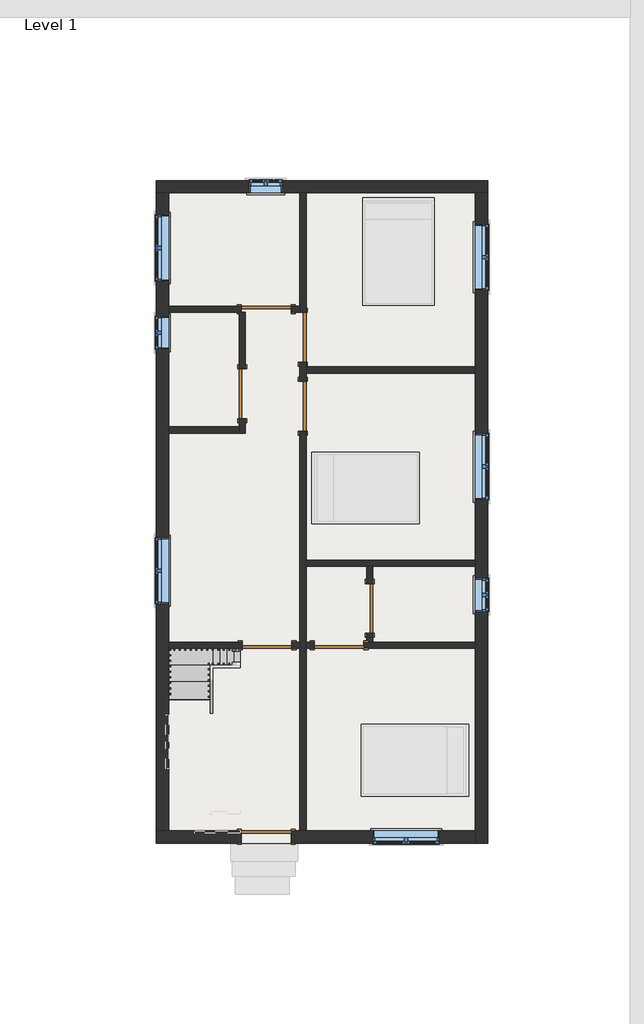
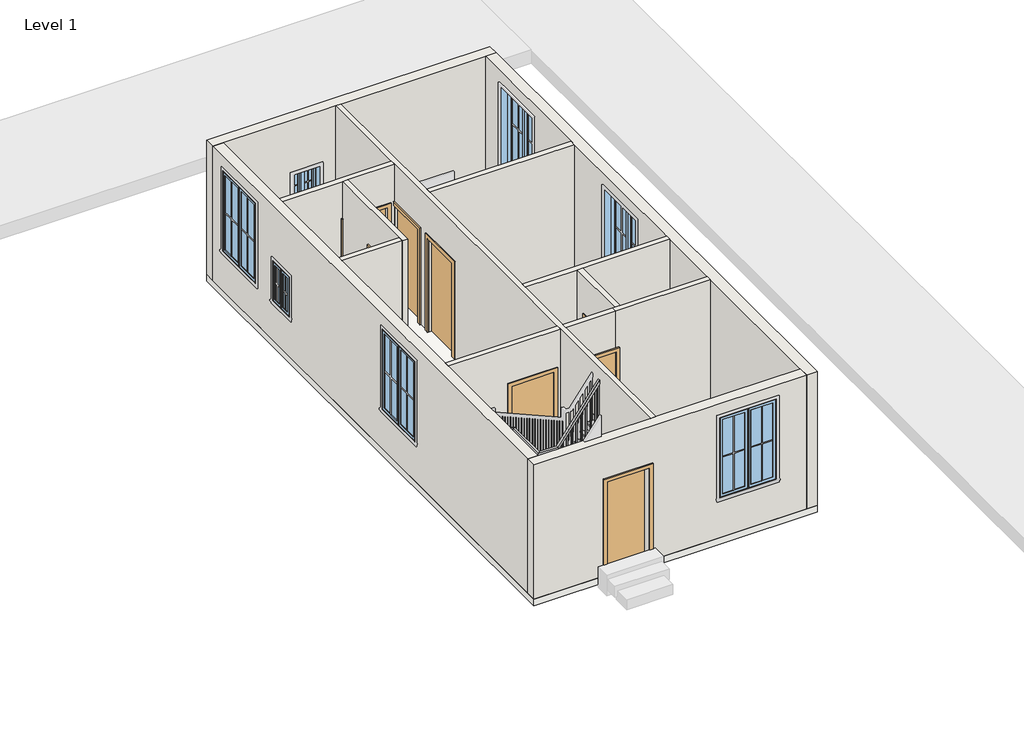
# One storey, part 1 of 2: 14 walls, 8 doors, 8 windows, 1 railing, 1 slab, 1 stair flight.
"""IFC4 building model written with IfcOpenShell, lengths in millimetres."""

from ifc_helpers import new_model, si_unit, frame, origin, origin_with_axes, place, context, project, spatial, polyline, outline, extrude, faceted_brep, transform, mapped, element, save
from components import door_e5f9f3c4, door_305aa2a5, door_a90ba1ad, stair_flight_0c8a4d61, window_c417fced, window_6ca1769e

model = new_model("IFC4")

# Units and contexts
model_context = context("Model", 3, world=origin())
ifc_project = project(units=[si_unit("LENGTHUNIT", "METRE", prefix="MILLI")], contexts=[model_context])

# Site, building, storey
site = spatial("IfcSite", under=ifc_project)
building = spatial("IfcBuilding", under=site)
storey = spatial("IfcBuildingStorey", under=building, Name="Level 1", Elevation=0.0)

# Doors
placement = place(None, origin())
door_shape = door_e5f9f3c4(model_context)
element("IfcDoor", 1, ObjectType="Single-Flush : 36\" x 84\"", at=placement, inside=storey, context=model_context, shape_type="MappedRepresentation", body=[
    mapped(door_shape, transform((3549.65, 11855.45, 0.0), x_axis=(1.0, 0.0, 0.0), y_axis=(0.0, 1.0, 0.0), z_axis=(0.0, 0.0, 1.0))),
])
element("IfcDoor", 2, ObjectType="Single-Flush : 36\" x 84\"", at=placement, inside=storey, context=model_context, shape_type="MappedRepresentation", body=[
    mapped(door_shape, transform((4222.75, 11341.1, 0.0), x_axis=(0.0, -1.0, 0.0), y_axis=(1.0, 0.0, 0.0), z_axis=(0.0, 0.0, 1.0))),
])
element("IfcDoor", 3, ObjectType="Single-Flush : 36\" x 84\"", at=placement, inside=storey, context=model_context, shape_type="MappedRepresentation", body=[
    mapped(door_shape, transform((5454.65, 6350.0, 0.0), x_axis=(0.0, -1.0, 0.0), y_axis=(1.0, 0.0, 0.0), z_axis=(0.0, 0.0, 1.0))),
])
element("IfcDoor", 4, ObjectType="Single-Flush : 36\" x 84\"", at=placement, inside=storey, context=model_context, shape_type="MappedRepresentation", body=[
    mapped(door_shape, transform((4889.5, 5670.55, 0.0), x_axis=(-1.0, 0.0, 0.0), y_axis=(0.0, -1.0, 0.0), z_axis=(0.0, 0.0, 1.0))),
])
door_2_shape = door_305aa2a5(model_context)
element("IfcDoor", 5, ObjectType="Single-Flush : 36\" x 84\"", at=placement, inside=storey, context=model_context, shape_type="MappedRepresentation", body=[
    mapped(door_2_shape, transform((3105.15, 10299.7, 0.0), x_axis=(0.0, -1.0, 0.0), y_axis=(1.0, 0.0, 0.0), z_axis=(0.0, 0.0, 1.0))),
])
element("IfcDoor", 6, ObjectType="Single-Flush : 36\" x 84\"", at=placement, inside=storey, context=model_context, shape_type="MappedRepresentation", body=[
    mapped(door_2_shape, transform((4222.75, 10071.1, 0.0), x_axis=(0.0, 1.0, 0.0), y_axis=(-1.0, 0.0, 0.0), z_axis=(0.0, 0.0, 1.0))),
])
element("IfcDoor", 7, ObjectType="Single-Flush : 36\" x 84\"", at=placement, inside=storey, context=model_context, shape_type="MappedRepresentation", body=[
    mapped(door_2_shape, transform((3562.35, 5670.55, 0.0), x_axis=(1.0, 0.0, 0.0), y_axis=(0.0, 1.0, 0.0), z_axis=(0.0, 0.0, 1.0))),
])
door_3_shape = door_a90ba1ad(model_context)
element("IfcDoor", 8, ObjectType="Single-Flush : 36\" x 84\"", at=placement, inside=storey, context=model_context, shape_type="MappedRepresentation", body=[
    mapped(door_3_shape, transform((3549.65, 2146.3, 0.0), x_axis=(-1.0, 0.0, 0.0), y_axis=(0.0, -1.0, 0.0), z_axis=(0.0, 0.0, 1.0))),
])

# Railing
element("IfcRailing", 9, ObjectType="Handrail - Rectangular", at=placement, inside=storey, context=model_context, shape_type="SolidModel", body=[
    faceted_brep([(3073.4, 5562.6, 1083.7333333), (3073.4, 5562.6, 999.0666667), (3073.4, 5613.4, 999.0666667), (3073.4, 5613.4, 1083.7333333), (2166.4083333, 5562.6, 2293.0555556), (2141.0083333, 5562.6, 2242.2555556), (2141.0083333, 5613.4, 2242.2555556), (2166.4083333, 5613.4, 2293.0555556), (1803.4, 5562.6, 2293.0555556), (1803.4, 5562.6, 2242.2555556), (1752.6, 5613.4, 2242.2555556), (1752.6, 5613.4, 2293.0555556), (1803.4, 4655.82, 2293.0555556), (1803.4, 4642.6563978, 2242.2555556), (1752.6, 4642.6563978, 2242.2555556), (1752.6, 4655.82, 2293.0555556), (1803.4, 3218.18, 3091.7444444), (1803.4, 3205.0163978, 3040.9444444), (1752.6, 3205.0163978, 3040.9444444), (1752.6, 3218.18, 3091.7444444), (1803.4, 2311.4, 3091.7444444), (1803.4, 2311.4, 3040.9444444), (1752.6, 2260.6, 3040.9444444), (1752.6, 2260.6, 3091.7444444), (2166.4083333, 2311.4, 3091.7444444), (2191.8083333, 2311.4, 3040.9444444), (2191.8083333, 2260.6, 3040.9444444), (2166.4083333, 2260.6, 3091.7444444), (3073.4, 2311.4, 4301.0666667), (3073.4, 2260.6, 4301.0666667), (3073.4, 2260.6, 4216.4), (3073.4, 2311.4, 4216.4)], [[[0, 1, 2, 3]], [[1, 0, 4, 5]], [[2, 1, 5, 6]], [[3, 2, 6, 7]], [[0, 3, 7, 4]], [[5, 4, 8, 9]], [[6, 5, 9, 10]], [[7, 6, 10, 11]], [[4, 7, 11, 8]], [[9, 8, 12, 13]], [[10, 9, 13, 14]], [[11, 10, 14, 15]], [[8, 11, 15, 12]], [[13, 12, 16, 17]], [[14, 13, 17, 18]], [[15, 14, 18, 19]], [[12, 15, 19, 16]], [[17, 16, 20, 21]], [[18, 17, 21, 22]], [[19, 18, 22, 23]], [[16, 19, 23, 20]], [[21, 20, 24, 25]], [[22, 21, 25, 26]], [[23, 22, 26, 27]], [[20, 23, 27, 24]], [[28, 29, 30, 31]], [[25, 24, 28, 31]], [[26, 25, 31, 30]], [[27, 26, 30, 29]], [[24, 27, 29, 28]]]),
    extrude(outline(polyline([(4127.5, 3006.725), (4102.1, 2987.675), (3217.3333333, 2987.675), (3217.3333333, 3006.725), (4127.5, 3006.725)])), frame((0.0, 2276.475, 0.0), z_axis=(0.0, 1.0, 0.0), x_axis=(0.0, 0.0, 1.0)), (0.0, 0.0, 1.0), 19.05),
    extrude(outline(polyline([(3992.0333333, 2905.125), (3966.6333333, 2886.075), (3048.0, 2886.075), (3048.0, 2905.125), (3992.0333333, 2905.125)])), frame((0.0, 2276.475, 0.0), z_axis=(0.0, 1.0, 0.0), x_axis=(0.0, 0.0, 1.0)), (0.0, 0.0, 1.0), 19.05),
    extrude(outline(polyline([(3856.5666667, 2803.525), (3831.1666667, 2784.475), (2878.6666667, 2784.475), (2878.6666667, 2803.525), (3856.5666667, 2803.525)])), frame((0.0, 2276.475, 0.0), z_axis=(0.0, 1.0, 0.0), x_axis=(0.0, 0.0, 1.0)), (0.0, 0.0, 1.0), 19.05),
    extrude(outline(polyline([(3721.1, 2701.925), (3695.7, 2682.875), (2878.6666667, 2682.875), (2878.6666667, 2701.925), (3721.1, 2701.925)])), frame((0.0, 2276.475, 0.0), z_axis=(0.0, 1.0, 0.0), x_axis=(0.0, 0.0, 1.0)), (0.0, 0.0, 1.0), 19.05),
    extrude(outline(polyline([(3585.6333333, 2600.325), (3560.2333333, 2581.275), (2709.3333333, 2581.275), (2709.3333333, 2600.325), (3585.6333333, 2600.325)])), frame((0.0, 2276.475, 0.0), z_axis=(0.0, 1.0, 0.0), x_axis=(0.0, 0.0, 1.0)), (0.0, 0.0, 1.0), 19.05),
    extrude(outline(polyline([(3450.1666667, 2498.725), (3424.7666667, 2479.675), (2540.0, 2479.675), (2540.0, 2498.725), (3450.1666667, 2498.725)])), frame((0.0, 2276.475, 0.0), z_axis=(0.0, 1.0, 0.0), x_axis=(0.0, 0.0, 1.0)), (0.0, 0.0, 1.0), 19.05),
    extrude(outline(polyline([(3314.7, 2397.125), (3289.3, 2378.075), (2540.0, 2378.075), (2540.0, 2397.125), (3314.7, 2397.125)])), frame((0.0, 2276.475, 0.0), z_axis=(0.0, 1.0, 0.0), x_axis=(0.0, 0.0, 1.0)), (0.0, 0.0, 1.0), 19.05),
    extrude(outline(polyline([(3179.2333333, 2295.525), (3153.8333333, 2276.475), (2540.0, 2276.475), (2540.0, 2295.525), (3179.2333333, 2295.525)])), frame((0.0, 2276.475, 0.0), z_axis=(0.0, 1.0, 0.0), x_axis=(0.0, 0.0, 1.0)), (0.0, 0.0, 1.0), 19.05),
    extrude(outline(polyline([(3043.7666667, 2193.925), (3018.3666667, 2174.875), (2540.0, 2174.875), (2540.0, 2193.925), (3043.7666667, 2193.925)])), frame((0.0, 2276.475, 0.0), z_axis=(0.0, 1.0, 0.0), x_axis=(0.0, 0.0, 1.0)), (0.0, 0.0, 1.0), 19.05),
    extrude(outline(polyline([(2073.275, 2276.475), (2073.275, 2295.525), (2092.325, 2295.525), (2092.325, 2276.475), (2073.275, 2276.475)])), frame((0.0, 0.0, 2540.0), z_axis=(0.0, 0.0, 1.0), x_axis=(1.0, 0.0, 0.0)), (0.0, 0.0, 1.0), 500.9444444),
    extrude(outline(polyline([(1971.675, 2276.475), (1971.675, 2295.525), (1990.725, 2295.525), (1990.725, 2276.475), (1971.675, 2276.475)])), frame((0.0, 0.0, 2540.0), z_axis=(0.0, 0.0, 1.0), x_axis=(1.0, 0.0, 0.0)), (0.0, 0.0, 1.0), 500.9444444),
    extrude(outline(polyline([(1870.075, 2276.475), (1870.075, 2295.525), (1889.125, 2295.525), (1889.125, 2276.475), (1870.075, 2276.475)])), frame((0.0, 0.0, 2540.0), z_axis=(0.0, 0.0, 1.0), x_axis=(1.0, 0.0, 0.0)), (0.0, 0.0, 1.0), 500.9444444),
    extrude(outline(polyline([(1768.475, 2346.325), (1787.525, 2346.325), (1787.525, 2327.275), (1768.475, 2327.275), (1768.475, 2346.325)])), frame((0.0, 0.0, 2540.0), z_axis=(0.0, 0.0, 1.0), x_axis=(1.0, 0.0, 0.0)), (0.0, 0.0, 1.0), 500.9444444),
    extrude(outline(polyline([(1768.475, 2447.925), (1787.525, 2447.925), (1787.525, 2428.875), (1768.475, 2428.875), (1768.475, 2447.925)])), frame((0.0, 0.0, 2540.0), z_axis=(0.0, 0.0, 1.0), x_axis=(1.0, 0.0, 0.0)), (0.0, 0.0, 1.0), 500.9444444),
    extrude(outline(polyline([(1768.475, 2549.525), (1787.525, 2549.525), (1787.525, 2530.475), (1768.475, 2530.475), (1768.475, 2549.525)])), frame((0.0, 0.0, 2540.0), z_axis=(0.0, 0.0, 1.0), x_axis=(1.0, 0.0, 0.0)), (0.0, 0.0, 1.0), 500.9444444),
    extrude(outline(polyline([(1768.475, 2651.125), (1787.525, 2651.125), (1787.525, 2632.075), (1768.475, 2632.075), (1768.475, 2651.125)])), frame((0.0, 0.0, 2370.6666667), z_axis=(0.0, 0.0, 1.0), x_axis=(1.0, 0.0, 0.0)), (0.0, 0.0, 1.0), 670.2777778),
    extrude(outline(polyline([(1768.475, 2752.725), (1787.525, 2752.725), (1787.525, 2733.675), (1768.475, 2733.675), (1768.475, 2752.725)])), frame((0.0, 0.0, 2370.6666667), z_axis=(0.0, 0.0, 1.0), x_axis=(1.0, 0.0, 0.0)), (0.0, 0.0, 1.0), 670.2777778),
    extrude(outline(polyline([(1768.475, 2854.325), (1787.525, 2854.325), (1787.525, 2835.275), (1768.475, 2835.275), (1768.475, 2854.325)])), frame((0.0, 0.0, 2370.6666667), z_axis=(0.0, 0.0, 1.0), x_axis=(1.0, 0.0, 0.0)), (0.0, 0.0, 1.0), 670.2777778),
    extrude(outline(polyline([(1768.475, 2955.925), (1787.525, 2955.925), (1787.525, 2936.875), (1768.475, 2936.875), (1768.475, 2955.925)])), frame((0.0, 0.0, 2201.3333333), z_axis=(0.0, 0.0, 1.0), x_axis=(1.0, 0.0, 0.0)), (0.0, 0.0, 1.0), 839.6111111),
    extrude(outline(polyline([(1768.475, 3057.525), (1787.525, 3057.525), (1787.525, 3038.475), (1768.475, 3038.475), (1768.475, 3057.525)])), frame((0.0, 0.0, 2201.3333333), z_axis=(0.0, 0.0, 1.0), x_axis=(1.0, 0.0, 0.0)), (0.0, 0.0, 1.0), 839.6111111),
    extrude(outline(polyline([(1768.475, 3159.125), (1787.525, 3159.125), (1787.525, 3140.075), (1768.475, 3140.075), (1768.475, 3159.125)])), frame((0.0, 0.0, 2201.3333333), z_axis=(0.0, 0.0, 1.0), x_axis=(1.0, 0.0, 0.0)), (0.0, 0.0, 1.0), 839.6111111),
    extrude(outline(polyline([(3241.675, 3020.5785543), (3260.725, 3009.995221), (3260.725, 2032.0), (3241.675, 2032.0), (3241.675, 3020.5785543)])), frame((1768.475, 0.0, 0.0), z_axis=(1.0, 0.0, 0.0), x_axis=(0.0, 1.0, 0.0)), (0.0, 0.0, 1.0), 19.05),
    extrude(outline(polyline([(3343.275, 2964.1341099), (3362.325, 2953.5507765), (3362.325, 2032.0), (3343.275, 2032.0), (3343.275, 2964.1341099)])), frame((1768.475, 0.0, 0.0), z_axis=(1.0, 0.0, 0.0), x_axis=(0.0, 1.0, 0.0)), (0.0, 0.0, 1.0), 19.05),
    extrude(outline(polyline([(3444.875, 2907.6896654), (3463.925, 2897.1063321), (3463.925, 2032.0), (3444.875, 2032.0), (3444.875, 2907.6896654)])), frame((1768.475, 0.0, 0.0), z_axis=(1.0, 0.0, 0.0), x_axis=(0.0, 1.0, 0.0)), (0.0, 0.0, 1.0), 19.05),
    extrude(outline(polyline([(3546.475, 2851.245221), (3565.525, 2840.6618876), (3565.525, 1862.6666667), (3546.475, 1862.6666667), (3546.475, 2851.245221)])), frame((1768.475, 0.0, 0.0), z_axis=(1.0, 0.0, 0.0), x_axis=(0.0, 1.0, 0.0)), (0.0, 0.0, 1.0), 19.05),
    extrude(outline(polyline([(3648.075, 2794.8007765), (3667.125, 2784.2174432), (3667.125, 1862.6666667), (3648.075, 1862.6666667), (3648.075, 2794.8007765)])), frame((1768.475, 0.0, 0.0), z_axis=(1.0, 0.0, 0.0), x_axis=(0.0, 1.0, 0.0)), (0.0, 0.0, 1.0), 19.05),
    extrude(outline(polyline([(3749.675, 2738.3563321), (3768.725, 2727.7729988), (3768.725, 1862.6666667), (3749.675, 1862.6666667), (3749.675, 2738.3563321)])), frame((1768.475, 0.0, 0.0), z_axis=(1.0, 0.0, 0.0), x_axis=(0.0, 1.0, 0.0)), (0.0, 0.0, 1.0), 19.05),
    extrude(outline(polyline([(3851.275, 2681.9118876), (3870.325, 2671.3285543), (3870.325, 1693.3333333), (3851.275, 1693.3333333), (3851.275, 2681.9118876)])), frame((1768.475, 0.0, 0.0), z_axis=(1.0, 0.0, 0.0), x_axis=(0.0, 1.0, 0.0)), (0.0, 0.0, 1.0), 19.05),
    extrude(outline(polyline([(3952.875, 2625.4674432), (3971.925, 2614.8841099), (3971.925, 1693.3333333), (3952.875, 1693.3333333), (3952.875, 2625.4674432)])), frame((1768.475, 0.0, 0.0), z_axis=(1.0, 0.0, 0.0), x_axis=(0.0, 1.0, 0.0)), (0.0, 0.0, 1.0), 19.05),
    extrude(outline(polyline([(4054.475, 2569.0229988), (4073.525, 2558.4396654), (4073.525, 1693.3333333), (4054.475, 1693.3333333), (4054.475, 2569.0229988)])), frame((1768.475, 0.0, 0.0), z_axis=(1.0, 0.0, 0.0), x_axis=(0.0, 1.0, 0.0)), (0.0, 0.0, 1.0), 19.05),
    extrude(outline(polyline([(4156.075, 2512.5785543), (4175.125, 2501.995221), (4175.125, 1524.0), (4156.075, 1524.0), (4156.075, 2512.5785543)])), frame((1768.475, 0.0, 0.0), z_axis=(1.0, 0.0, 0.0), x_axis=(0.0, 1.0, 0.0)), (0.0, 0.0, 1.0), 19.05),
    extrude(outline(polyline([(4257.675, 2456.1341099), (4276.725, 2445.5507765), (4276.725, 1524.0), (4257.675, 1524.0), (4257.675, 2456.1341099)])), frame((1768.475, 0.0, 0.0), z_axis=(1.0, 0.0, 0.0), x_axis=(0.0, 1.0, 0.0)), (0.0, 0.0, 1.0), 19.05),
    extrude(outline(polyline([(4359.275, 2399.6896654), (4378.325, 2389.1063321), (4378.325, 1524.0), (4359.275, 1524.0), (4359.275, 2399.6896654)])), frame((1768.475, 0.0, 0.0), z_axis=(1.0, 0.0, 0.0), x_axis=(0.0, 1.0, 0.0)), (0.0, 0.0, 1.0), 19.05),
    extrude(outline(polyline([(4460.875, 2343.245221), (4479.925, 2332.6618876), (4479.925, 1354.6666667), (4460.875, 1354.6666667), (4460.875, 2343.245221)])), frame((1768.475, 0.0, 0.0), z_axis=(1.0, 0.0, 0.0), x_axis=(0.0, 1.0, 0.0)), (0.0, 0.0, 1.0), 19.05),
    extrude(outline(polyline([(4562.475, 2286.8007765), (4581.525, 2276.2174432), (4581.525, 1354.6666667), (4562.475, 1354.6666667), (4562.475, 2286.8007765)])), frame((1768.475, 0.0, 0.0), z_axis=(1.0, 0.0, 0.0), x_axis=(0.0, 1.0, 0.0)), (0.0, 0.0, 1.0), 19.05),
    extrude(outline(polyline([(1768.475, 4683.125), (1787.525, 4683.125), (1787.525, 4664.075), (1768.475, 4664.075), (1768.475, 4683.125)])), frame((0.0, 0.0, 1354.6666667), z_axis=(0.0, 0.0, 1.0), x_axis=(1.0, 0.0, 0.0)), (0.0, 0.0, 1.0), 887.5888889),
    extrude(outline(polyline([(1768.475, 4784.725), (1787.525, 4784.725), (1787.525, 4765.675), (1768.475, 4765.675), (1768.475, 4784.725)])), frame((0.0, 0.0, 1185.3333333), z_axis=(0.0, 0.0, 1.0), x_axis=(1.0, 0.0, 0.0)), (0.0, 0.0, 1.0), 1056.9222222),
    extrude(outline(polyline([(1768.475, 4886.325), (1787.525, 4886.325), (1787.525, 4867.275), (1768.475, 4867.275), (1768.475, 4886.325)])), frame((0.0, 0.0, 1185.3333333), z_axis=(0.0, 0.0, 1.0), x_axis=(1.0, 0.0, 0.0)), (0.0, 0.0, 1.0), 1056.9222222),
    extrude(outline(polyline([(1768.475, 4987.925), (1787.525, 4987.925), (1787.525, 4968.875), (1768.475, 4968.875), (1768.475, 4987.925)])), frame((0.0, 0.0, 1185.3333333), z_axis=(0.0, 0.0, 1.0), x_axis=(1.0, 0.0, 0.0)), (0.0, 0.0, 1.0), 1056.9222222),
    extrude(outline(polyline([(1768.475, 5089.525), (1787.525, 5089.525), (1787.525, 5070.475), (1768.475, 5070.475), (1768.475, 5089.525)])), frame((0.0, 0.0, 1016.0), z_axis=(0.0, 0.0, 1.0), x_axis=(1.0, 0.0, 0.0)), (0.0, 0.0, 1.0), 1226.2555556),
    extrude(outline(polyline([(1768.475, 5191.125), (1787.525, 5191.125), (1787.525, 5172.075), (1768.475, 5172.075), (1768.475, 5191.125)])), frame((0.0, 0.0, 1016.0), z_axis=(0.0, 0.0, 1.0), x_axis=(1.0, 0.0, 0.0)), (0.0, 0.0, 1.0), 1226.2555556),
    extrude(outline(polyline([(1768.475, 5292.725), (1787.525, 5292.725), (1787.525, 5273.675), (1768.475, 5273.675), (1768.475, 5292.725)])), frame((0.0, 0.0, 1016.0), z_axis=(0.0, 0.0, 1.0), x_axis=(1.0, 0.0, 0.0)), (0.0, 0.0, 1.0), 1226.2555556),
    extrude(outline(polyline([(1768.475, 5394.325), (1787.525, 5394.325), (1787.525, 5375.275), (1768.475, 5375.275), (1768.475, 5394.325)])), frame((0.0, 0.0, 846.6666667), z_axis=(0.0, 0.0, 1.0), x_axis=(1.0, 0.0, 0.0)), (0.0, 0.0, 1.0), 1395.5888889),
    extrude(outline(polyline([(1768.475, 5495.925), (1787.525, 5495.925), (1787.525, 5476.875), (1768.475, 5476.875), (1768.475, 5495.925)])), frame((0.0, 0.0, 846.6666667), z_axis=(0.0, 0.0, 1.0), x_axis=(1.0, 0.0, 0.0)), (0.0, 0.0, 1.0), 1395.5888889),
    extrude(outline(polyline([(1863.725, 5597.525), (1863.725, 5578.475), (1844.675, 5578.475), (1844.675, 5597.525), (1863.725, 5597.525)])), frame((0.0, 0.0, 846.6666667), z_axis=(0.0, 0.0, 1.0), x_axis=(1.0, 0.0, 0.0)), (0.0, 0.0, 1.0), 1395.5888889),
    extrude(outline(polyline([(1965.325, 5597.525), (1965.325, 5578.475), (1946.275, 5578.475), (1946.275, 5597.525), (1965.325, 5597.525)])), frame((0.0, 0.0, 846.6666667), z_axis=(0.0, 0.0, 1.0), x_axis=(1.0, 0.0, 0.0)), (0.0, 0.0, 1.0), 1395.5888889),
    extrude(outline(polyline([(2066.925, 5597.525), (2066.925, 5578.475), (2047.875, 5578.475), (2047.875, 5597.525), (2066.925, 5597.525)])), frame((0.0, 0.0, 846.6666667), z_axis=(0.0, 0.0, 1.0), x_axis=(1.0, 0.0, 0.0)), (0.0, 0.0, 1.0), 1395.5888889),
    extrude(outline(polyline([(2168.525, 5597.525), (2168.525, 5578.475), (2149.475, 5578.475), (2149.475, 5597.525), (2168.525, 5597.525)])), frame((0.0, 0.0, 846.6666667), z_axis=(0.0, 0.0, 1.0), x_axis=(1.0, 0.0, 0.0)), (0.0, 0.0, 1.0), 1395.5888889),
    extrude(outline(polyline([(2070.1, 2270.125), (2095.5, 2251.075), (846.6666667, 2251.075), (846.6666667, 2270.125), (2070.1, 2270.125)])), frame((0.0, 5578.475, 0.0), z_axis=(0.0, 1.0, 0.0), x_axis=(0.0, 0.0, 1.0)), (0.0, 0.0, 1.0), 19.05),
    extrude(outline(polyline([(1934.6333333, 2371.725), (1960.0333333, 2352.675), (846.6666667, 2352.675), (846.6666667, 2371.725), (1934.6333333, 2371.725)])), frame((0.0, 5578.475, 0.0), z_axis=(0.0, 1.0, 0.0), x_axis=(0.0, 0.0, 1.0)), (0.0, 0.0, 1.0), 19.05),
    extrude(outline(polyline([(1799.1666667, 2473.325), (1824.5666667, 2454.275), (846.6666667, 2454.275), (846.6666667, 2473.325), (1799.1666667, 2473.325)])), frame((0.0, 5578.475, 0.0), z_axis=(0.0, 1.0, 0.0), x_axis=(0.0, 0.0, 1.0)), (0.0, 0.0, 1.0), 19.05),
    extrude(outline(polyline([(1663.7, 2574.925), (1689.1, 2555.875), (846.6666667, 2555.875), (846.6666667, 2574.925), (1663.7, 2574.925)])), frame((0.0, 5578.475, 0.0), z_axis=(0.0, 1.0, 0.0), x_axis=(0.0, 0.0, 1.0)), (0.0, 0.0, 1.0), 19.05),
    extrude(outline(polyline([(1528.2333333, 2676.525), (1553.6333333, 2657.475), (677.3333333, 2657.475), (677.3333333, 2676.525), (1528.2333333, 2676.525)])), frame((0.0, 5578.475, 0.0), z_axis=(0.0, 1.0, 0.0), x_axis=(0.0, 0.0, 1.0)), (0.0, 0.0, 1.0), 19.05),
    extrude(outline(polyline([(1392.7666667, 2778.125), (1418.1666667, 2759.075), (508.0, 2759.075), (508.0, 2778.125), (1392.7666667, 2778.125)])), frame((0.0, 5578.475, 0.0), z_axis=(0.0, 1.0, 0.0), x_axis=(0.0, 0.0, 1.0)), (0.0, 0.0, 1.0), 19.05),
    extrude(outline(polyline([(1257.3, 2879.725), (1282.7, 2860.675), (338.6666667, 2860.675), (338.6666667, 2879.725), (1257.3, 2879.725)])), frame((0.0, 5578.475, 0.0), z_axis=(0.0, 1.0, 0.0), x_axis=(0.0, 0.0, 1.0)), (0.0, 0.0, 1.0), 19.05),
    extrude(outline(polyline([(1121.8333333, 2981.325), (1147.2333333, 2962.275), (169.3333333, 2962.275), (169.3333333, 2981.325), (1121.8333333, 2981.325)])), frame((0.0, 5578.475, 0.0), z_axis=(0.0, 1.0, 0.0), x_axis=(0.0, 0.0, 1.0)), (0.0, 0.0, 1.0), 19.05),
    extrude(outline(polyline([(1768.475, 2295.525), (1787.525, 2295.525), (1787.525, 2276.475), (1768.475, 2276.475), (1768.475, 2295.525)])), frame((0.0, 0.0, 2540.0), z_axis=(0.0, 0.0, 1.0), x_axis=(1.0, 0.0, 0.0)), (0.0, 0.0, 1.0), 500.9444444),
    extrude(outline(polyline([(1787.525, 5597.525), (1787.525, 5578.475), (1768.475, 5578.475), (1768.475, 5597.525), (1787.525, 5597.525)])), frame((0.0, 0.0, 846.6666667), z_axis=(0.0, 0.0, 1.0), x_axis=(1.0, 0.0, 0.0)), (0.0, 0.0, 1.0), 1395.5888889),
    extrude(outline(polyline([(4216.4, 3073.4), (4191.0, 3054.35), (3217.3333333, 3054.35), (3217.3333333, 3073.4), (4216.4, 3073.4)])), frame((0.0, 2276.475, 0.0), z_axis=(0.0, 1.0, 0.0), x_axis=(0.0, 0.0, 1.0)), (0.0, 0.0, 1.0), 19.05),
    extrude(outline(polyline([(999.0666667, 3073.4), (1024.4666667, 3054.35), (169.3333333, 3054.35), (169.3333333, 3073.4), (999.0666667, 3073.4)])), frame((0.0, 5578.475, 0.0), z_axis=(0.0, 1.0, 0.0), x_axis=(0.0, 0.0, 1.0)), (0.0, 0.0, 1.0), 19.05),
])

# Slab
element("IfcSlab", 10, ObjectType="Generic - 12\"", at=placement, inside=storey, context=model_context, shape_type="SweptSolid", body=[
    extrude(outline(polyline([(7620.0, 14224.0), (7620.0, 2032.0), (1524.0, 2032.0), (1524.0, 14224.0), (7620.0, 14224.0)])), frame((0.0, 0.0, -152.4), z_axis=(0.0, 0.0, 1.0), x_axis=(1.0, 0.0, 0.0)), (0.0, 0.0, 1.0), 152.4),
])

# Stair flight
stair_flight_shape = stair_flight_0c8a4d61(model_context)
element("IfcStairFlight", 11, ObjectType="2\" Tread 1\" Nosing 1/4\" Riser", at=placement, inside=storey, context=model_context, shape_type="MappedRepresentation", body=[
    mapped(stair_flight_shape, transform((0.0, 0.0, 0.0), x_axis=(1.0, 0.0, 0.0), y_axis=(0.0, 1.0, 0.0), z_axis=(0.0, 0.0, 1.0))),
])

# Walls
element("IfcWall", 12, ObjectType="Generic - 5\"", at=placement, inside=storey, context=model_context, shape_type="Brep", body=[
    faceted_brep([(4165.6, 10883.9, 0.0), (4165.6, 10528.3, 0.0), (4165.6, 10528.3, 2133.6), (4165.6, 9613.9, 2133.6), (4165.6, 9613.9, 0.0), (4165.6, 5727.7, 0.0), (4165.6, 5613.4, 0.0), (4165.6, 2260.6, 0.0), (4165.6, 2260.6, 3048.0), (4165.6, 5613.4, 3048.0), (4165.6, 5727.7, 3048.0), (4165.6, 11798.3, 3048.0), (4165.6, 11912.6, 3048.0), (4165.6, 13995.4, 3048.0), (4165.6, 13995.4, 0.0), (4165.6, 11912.6, 0.0), (4165.6, 11798.3, 0.0), (4165.6, 11798.3, 2133.6), (4165.6, 10883.9, 2133.6), (4279.9, 10528.3, 2133.6), (4279.9, 10528.3, 0.0), (4279.9, 10680.7, 0.0), (4279.9, 10795.0, 0.0), (4279.9, 10883.9, 0.0), (4279.9, 10883.9, 2133.6), (4279.9, 11798.3, 2133.6), (4279.9, 11798.3, 0.0), (4279.9, 13995.4, 0.0), (4279.9, 13995.4, 3048.0), (4279.9, 10795.0, 3048.0), (4279.9, 10680.7, 3048.0), (4279.9, 7239.0, 3048.0), (4279.9, 7124.7, 3048.0), (4279.9, 5727.7, 3048.0), (4279.9, 5613.4, 3048.0), (4279.9, 2260.6, 3048.0), (4279.9, 2260.6, 0.0), (4279.9, 5613.4, 0.0), (4279.9, 5727.7, 0.0), (4279.9, 7124.7, 0.0), (4279.9, 7239.0, 0.0), (4279.9, 9613.9, 0.0), (4279.9, 9613.9, 2133.6)], [[[0, 1, 2, 3, 4, 5, 6, 7, 8, 9, 10, 11, 12, 13, 14, 15, 16, 17, 18]], [[19, 20, 21, 22, 23, 24, 25, 26, 27, 28, 29, 30, 31, 32, 33, 34, 35, 36, 37, 38, 39, 40, 41, 42]], [[16, 15, 14, 27, 26]], [[41, 40, 39, 38, 37, 36, 7, 6, 5, 4]], [[23, 22, 21, 20, 1, 0]], [[13, 12, 11, 10, 9, 8, 35, 34, 33, 32, 31, 30, 29, 28]], [[14, 13, 28, 27]], [[8, 7, 36, 35]], [[24, 23, 0, 18]], [[25, 24, 18, 17]], [[26, 25, 17, 16]], [[2, 1, 20, 19]], [[3, 2, 19, 42]], [[4, 3, 42, 41]]]),
])
element("IfcWall", 13, ObjectType="Generic - 5\"", at=placement, inside=storey, context=model_context, shape_type="Brep", body=[
    faceted_brep([(4279.9, 7124.7, 0.0), (5397.5, 7124.7, 0.0), (5511.8, 7124.7, 0.0), (7391.4, 7124.7, 0.0), (7391.4, 7124.7, 3048.0), (5511.8, 7124.7, 3048.0), (5397.5, 7124.7, 3048.0), (4279.9, 7124.7, 3048.0), (4279.9, 7239.0, 0.0), (4279.9, 7239.0, 3048.0), (7391.4, 7239.0, 3048.0), (7391.4, 7239.0, 0.0)], [[[0, 1, 2, 3, 4, 5, 6, 7]], [[8, 9, 10, 11]], [[3, 2, 1, 0, 8, 11]], [[7, 6, 5, 4, 10, 9]], [[4, 3, 11, 10]], [[0, 7, 9, 8]]]),
])
element("IfcWall", 14, ObjectType="Generic - 5\"", at=placement, inside=storey, context=model_context, shape_type="SweptSolid", body=[
    extrude(outline(polyline([(5892.8, 2133.6), (5892.8, 0.0), (5727.7, 0.0), (5727.7, 3048.0), (7124.7, 3048.0), (7124.7, 0.0), (6807.2, 0.0), (6807.2, 2133.6), (5892.8, 2133.6)])), frame((5397.5, 0.0, 0.0), z_axis=(1.0, 0.0, 0.0), x_axis=(0.0, 1.0, 0.0)), (0.0, 0.0, 1.0), 114.3),
])
element("IfcWall", 15, ObjectType="Generic - 5\"", at=placement, inside=storey, context=model_context, shape_type="Brep", body=[
    faceted_brep([(7391.4, 5727.7, 0.0), (5511.8, 5727.7, 0.0), (5397.5, 5727.7, 0.0), (5346.7, 5727.7, 0.0), (5346.7, 5727.7, 2133.6), (5346.7, 5727.7, 3048.0), (5397.5, 5727.7, 3048.0), (5511.8, 5727.7, 3048.0), (7391.4, 5727.7, 3048.0), (7391.4, 5613.4, 0.0), (7391.4, 5613.4, 3048.0), (5346.7, 5613.4, 3048.0), (5346.7, 5613.4, 2133.6), (5346.7, 5613.4, 0.0)], [[[0, 1, 2, 3, 4, 5, 6, 7, 8]], [[9, 10, 11, 12, 13]], [[3, 2, 1, 0, 9, 13]], [[5, 4, 3, 13, 12, 11]], [[8, 7, 6, 5, 11, 10]], [[0, 8, 10, 9]]]),
])
element("IfcWall", 16, ObjectType="Generic - 5\"", at=placement, inside=storey, context=model_context, shape_type="SweptSolid", body=[
    extrude(outline(polyline([(7391.4, 10680.7), (4279.9, 10680.7), (4279.9, 10795.0), (7391.4, 10795.0), (7391.4, 10680.7)])), origin_with_axes(), (0.0, 0.0, 1.0), 3048.0),
])
element("IfcWall", 17, ObjectType="Generic - 5\"", at=placement, inside=storey, context=model_context, shape_type="Brep", body=[
    faceted_brep([(4006.85, 11798.3, 2133.6), (4006.85, 11798.3, 0.0), (4165.6, 11798.3, 0.0), (4165.6, 11798.3, 3048.0), (3162.3, 11798.3, 3048.0), (3048.0, 11798.3, 3048.0), (1752.6, 11798.3, 3048.0), (1752.6, 11798.3, 0.0), (3048.0, 11798.3, 0.0), (3092.45, 11798.3, 0.0), (3092.45, 11798.3, 2133.6), (4165.6, 11912.6, 0.0), (4006.85, 11912.6, 0.0), (4006.85, 11912.6, 2133.6), (3092.45, 11912.6, 2133.6), (3092.45, 11912.6, 0.0), (1752.6, 11912.6, 0.0), (1752.6, 11912.6, 3048.0), (4165.6, 11912.6, 3048.0)], [[[0, 1, 2, 3, 4, 5, 6, 7, 8, 9, 10]], [[11, 12, 13, 14, 15, 16, 17, 18]], [[2, 1, 12, 11]], [[9, 8, 7, 16, 15]], [[6, 5, 4, 3, 18, 17]], [[7, 6, 17, 16]], [[3, 2, 11, 18]], [[13, 12, 1, 0]], [[14, 13, 0, 10]], [[15, 14, 10, 9]]]),
])
element("IfcWall", 18, ObjectType="Generic - 5\"", at=placement, inside=storey, context=model_context, shape_type="Brep", body=[
    faceted_brep([(3048.0, 9842.5, 2133.6), (3048.0, 9842.5, 0.0), (3048.0, 9690.1, 0.0), (3048.0, 9575.8, 0.0), (3048.0, 9575.8, 3048.0), (3048.0, 9690.1, 3048.0), (3048.0, 11798.3, 3048.0), (3048.0, 11798.3, 0.0), (3048.0, 10756.9, 0.0), (3048.0, 10756.9, 2133.6), (3162.3, 9575.8, 0.0), (3162.3, 9842.5, 0.0), (3162.3, 9842.5, 2133.6), (3162.3, 10756.9, 2133.6), (3162.3, 10756.9, 0.0), (3162.3, 11798.3, 0.0), (3162.3, 11798.3, 3048.0), (3162.3, 9575.8, 3048.0), (3092.45, 11798.3, 0.0)], [[[0, 1, 2, 3, 4, 5, 6, 7, 8, 9]], [[10, 11, 12, 13, 14, 15, 16, 17]], [[8, 7, 18, 15, 14]], [[3, 2, 1, 11, 10]], [[6, 5, 4, 17, 16]], [[7, 6, 16, 15, 18]], [[4, 3, 10, 17]], [[12, 11, 1, 0]], [[13, 12, 0, 9]], [[14, 13, 9, 8]]]),
])
element("IfcWall", 19, ObjectType="Generic - 5\"", at=placement, inside=storey, context=model_context, shape_type="SweptSolid", body=[
    extrude(outline(polyline([(1752.6, 9690.1), (3048.0, 9690.1), (3048.0, 9575.8), (1752.6, 9575.8), (1752.6, 9690.1)])), origin_with_axes(), (0.0, 0.0, 1.0), 3048.0),
])
element("IfcWall", 20, ObjectType="Generic - 5\"", at=placement, inside=storey, context=model_context, shape_type="SweptSolid", body=[
    extrude(outline(polyline([(2133.6, 4019.55), (0.0, 4019.55), (0.0, 4165.6), (3048.0, 4165.6), (3048.0, 1752.6), (0.0, 1752.6), (0.0, 3105.15), (2133.6, 3105.15), (2133.6, 4019.55)])), frame((0.0, 5613.4, 0.0), z_axis=(0.0, 1.0, 0.0), x_axis=(0.0, 0.0, 1.0)), (0.0, 0.0, 1.0), 114.3),
])
element("IfcWall", 21, ObjectType="Generic - 5\"", at=placement, inside=storey, context=model_context, shape_type="SweptSolid", body=[
    extrude(outline(polyline([(3048.0, 5346.7), (3048.0, 4279.9), (0.0, 4279.9), (0.0, 4432.3), (2133.6, 4432.3), (2133.6, 5346.7), (3048.0, 5346.7)])), frame((0.0, 5613.4, 0.0), z_axis=(0.0, 1.0, 0.0), x_axis=(0.0, 0.0, 1.0)), (0.0, 0.0, 1.0), 114.3),
])
element("IfcWall", 22, ObjectType="Generic - 8\"", at=placement, inside=storey, context=model_context, shape_type="Brep", body=[
    faceted_brep([(1524.0, 13995.4, 0.0), (1752.6, 13995.4, 0.0), (4165.6, 13995.4, 0.0), (4279.9, 13995.4, 0.0), (7391.4, 13995.4, 0.0), (7620.0, 13995.4, 0.0), (7620.0, 13995.4, 3048.0), (7391.4, 13995.4, 3048.0), (4279.9, 13995.4, 3048.0), (4165.6, 13995.4, 3048.0), (1752.6, 13995.4, 3048.0), (1524.0, 13995.4, 3048.0), (3841.75, 13995.4, 1828.8), (3841.75, 13995.4, 914.4), (3232.15, 13995.4, 914.4), (3232.15, 13995.4, 1828.8), (1524.0, 14224.0, 0.0), (1524.0, 14224.0, 3048.0), (7620.0, 14224.0, 3048.0), (7620.0, 14224.0, 0.0), (3841.75, 14224.0, 1828.8), (3232.15, 14224.0, 1828.8), (3232.15, 14224.0, 914.4), (3841.75, 14224.0, 914.4)], [[[0, 1, 2, 3, 4, 5, 6, 7, 8, 9, 10, 11], [12, 13, 14, 15]], [[16, 17, 18, 19], [20, 21, 22, 23]], [[5, 4, 3, 2, 1, 0, 16, 19]], [[6, 5, 19, 18]], [[0, 11, 17, 16]], [[11, 10, 9, 8, 7, 6, 18, 17]], [[13, 12, 20, 23]], [[14, 13, 23, 22]], [[15, 14, 22, 21]], [[12, 15, 21, 20]]]),
])
element("IfcWall", 23, ObjectType="Generic - 8\"", at=placement, inside=storey, context=model_context, shape_type="Brep", body=[
    faceted_brep([(7391.4, 13995.4, 0.0), (7391.4, 10795.0, 0.0), (7391.4, 10680.7, 0.0), (7391.4, 7239.0, 0.0), (7391.4, 7124.7, 0.0), (7391.4, 5727.7, 0.0), (7391.4, 5613.4, 0.0), (7391.4, 2260.6, 0.0), (7391.4, 2032.0, 0.0), (7391.4, 2032.0, 3048.0), (7391.4, 2260.6, 3048.0), (7391.4, 5613.4, 3048.0), (7391.4, 5727.7, 3048.0), (7391.4, 7124.7, 3048.0), (7391.4, 7239.0, 3048.0), (7391.4, 10680.7, 3048.0), (7391.4, 10795.0, 3048.0), (7391.4, 13995.4, 3048.0), (7391.4, 12204.7, 2743.2), (7391.4, 12204.7, 914.4), (7391.4, 13423.9, 914.4), (7391.4, 13423.9, 2743.2), (7391.4, 8350.25, 2743.2), (7391.4, 8350.25, 914.4), (7391.4, 9569.45, 914.4), (7391.4, 9569.45, 2743.2), (7391.4, 6292.85, 1828.8), (7391.4, 6292.85, 914.4), (7391.4, 6902.45, 914.4), (7391.4, 6902.45, 1828.8), (7620.0, 13995.4, 0.0), (7620.0, 13995.4, 3048.0), (7620.0, 2032.0, 3048.0), (7620.0, 2032.0, 0.0), (7620.0, 12204.7, 2743.2), (7620.0, 13423.9, 2743.2), (7620.0, 13423.9, 914.4), (7620.0, 12204.7, 914.4), (7620.0, 8350.25, 2743.2), (7620.0, 9569.45, 2743.2), (7620.0, 9569.45, 914.4), (7620.0, 8350.25, 914.4), (7620.0, 6292.85, 1828.8), (7620.0, 6902.45, 1828.8), (7620.0, 6902.45, 914.4), (7620.0, 6292.85, 914.4)], [[[0, 1, 2, 3, 4, 5, 6, 7, 8, 9, 10, 11, 12, 13, 14, 15, 16, 17], [18, 19, 20, 21], [22, 23, 24, 25], [26, 27, 28, 29]], [[30, 31, 32, 33], [34, 35, 36, 37], [38, 39, 40, 41], [42, 43, 44, 45]], [[8, 7, 6, 5, 4, 3, 2, 1, 0, 30, 33]], [[0, 17, 31, 30]], [[9, 8, 33, 32]], [[17, 16, 15, 14, 13, 12, 11, 10, 9, 32, 31]], [[19, 18, 34, 37]], [[20, 19, 37, 36]], [[21, 20, 36, 35]], [[18, 21, 35, 34]], [[23, 22, 38, 41]], [[24, 23, 41, 40]], [[25, 24, 40, 39]], [[22, 25, 39, 38]], [[27, 26, 42, 45]], [[28, 27, 45, 44]], [[29, 28, 44, 43]], [[26, 29, 43, 42]]]),
])
element("IfcWall", 24, ObjectType="Generic - 8\"", at=placement, inside=storey, context=model_context, shape_type="Brep", body=[
    faceted_brep([(3092.45, 2260.6, 2133.6), (3092.45, 2260.6, 0.0), (1752.6, 2260.6, 0.0), (1524.0, 2260.6, 0.0), (1524.0, 2260.6, 3048.0), (1752.6, 2260.6, 3048.0), (4165.6, 2260.6, 3048.0), (4279.9, 2260.6, 3048.0), (7391.4, 2260.6, 3048.0), (7391.4, 2260.6, 0.0), (4279.9, 2260.6, 0.0), (4165.6, 2260.6, 0.0), (4006.85, 2260.6, 0.0), (4006.85, 2260.6, 2133.6), (5511.8, 2260.6, 2743.2), (5511.8, 2260.6, 914.4), (6731.0, 2260.6, 914.4), (6731.0, 2260.6, 2743.2), (1524.0, 2032.0, 0.0), (3092.45, 2032.0, 0.0), (3092.45, 2032.0, 2133.6), (4006.85, 2032.0, 2133.6), (4006.85, 2032.0, 0.0), (7391.4, 2032.0, 0.0), (7391.4, 2032.0, 3048.0), (1524.0, 2032.0, 3048.0), (5511.8, 2032.0, 2743.2), (6731.0, 2032.0, 2743.2), (6731.0, 2032.0, 914.4), (5511.8, 2032.0, 914.4)], [[[0, 1, 2, 3, 4, 5, 6, 7, 8, 9, 10, 11, 12, 13], [14, 15, 16, 17]], [[18, 19, 20, 21, 22, 23, 24, 25], [26, 27, 28, 29]], [[3, 2, 1, 19, 18]], [[12, 11, 10, 9, 23, 22]], [[9, 8, 24, 23]], [[4, 3, 18, 25]], [[8, 7, 6, 5, 4, 25, 24]], [[20, 19, 1, 0]], [[21, 20, 0, 13]], [[22, 21, 13, 12]], [[15, 14, 26, 29]], [[16, 15, 29, 28]], [[17, 16, 28, 27]], [[14, 17, 27, 26]]]),
])
element("IfcWall", 25, ObjectType="Generic - 8\"", at=placement, inside=storey, context=model_context, shape_type="Brep", body=[
    faceted_brep([(1752.6, 2260.6, 0.0), (1752.6, 5613.4, 0.0), (1752.6, 5727.7, 0.0), (1752.6, 9575.8, 0.0), (1752.6, 9690.1, 0.0), (1752.6, 11798.3, 0.0), (1752.6, 11912.6, 0.0), (1752.6, 13995.4, 0.0), (1752.6, 13995.4, 3048.0), (1752.6, 11912.6, 3048.0), (1752.6, 11798.3, 3048.0), (1752.6, 9690.1, 3048.0), (1752.6, 9575.8, 3048.0), (1752.6, 5727.7, 3048.0), (1752.6, 5613.4, 3048.0), (1752.6, 2260.6, 3048.0), (1752.6, 13592.175, 2743.2), (1752.6, 13592.175, 914.4), (1752.6, 12372.975, 914.4), (1752.6, 12372.975, 2743.2), (1752.6, 7651.75, 2743.2), (1752.6, 7651.75, 914.4), (1752.6, 6432.55, 914.4), (1752.6, 6432.55, 2743.2), (1752.6, 11728.45, 1828.8), (1752.6, 11728.45, 914.4), (1752.6, 11118.85, 914.4), (1752.6, 11118.85, 1828.8), (1524.0, 2260.6, 0.0), (1524.0, 2260.6, 3048.0), (1524.0, 13995.4, 3048.0), (1524.0, 13995.4, 0.0), (1524.0, 13592.175, 2743.2), (1524.0, 12372.975, 2743.2), (1524.0, 12372.975, 914.4), (1524.0, 13592.175, 914.4), (1524.0, 7651.75, 2743.2), (1524.0, 6432.55, 2743.2), (1524.0, 6432.55, 914.4), (1524.0, 7651.75, 914.4), (1524.0, 11728.45, 1828.8), (1524.0, 11118.85, 1828.8), (1524.0, 11118.85, 914.4), (1524.0, 11728.45, 914.4)], [[[0, 1, 2, 3, 4, 5, 6, 7, 8, 9, 10, 11, 12, 13, 14, 15], [16, 17, 18, 19], [20, 21, 22, 23], [24, 25, 26, 27]], [[28, 29, 30, 31], [32, 33, 34, 35], [36, 37, 38, 39], [40, 41, 42, 43]], [[7, 6, 5, 4, 3, 2, 1, 0, 28, 31]], [[8, 7, 31, 30]], [[0, 15, 29, 28]], [[15, 14, 13, 12, 11, 10, 9, 8, 30, 29]], [[17, 16, 32, 35]], [[18, 17, 35, 34]], [[19, 18, 34, 33]], [[16, 19, 33, 32]], [[21, 20, 36, 39]], [[22, 21, 39, 38]], [[23, 22, 38, 37]], [[20, 23, 37, 36]], [[25, 24, 40, 43]], [[26, 25, 43, 42]], [[27, 26, 42, 41]], [[24, 27, 41, 40]]]),
])

# Windows
window_shape = window_c417fced(model_context)
element("IfcWindow", 26, ObjectType="Window-Casement-Double : 24\" x 36\"", at=placement, inside=storey, context=model_context, shape_type="MappedRepresentation", body=[
    mapped(window_shape, transform((7505.7, 6597.65, 0.0), x_axis=(0.0, -1.0, 0.0), y_axis=(1.0, 0.0, 0.0), z_axis=(0.0, 0.0, 1.0))),
])
element("IfcWindow", 27, ObjectType="Window-Casement-Double : 24\" x 36\"", at=placement, inside=storey, context=model_context, shape_type="MappedRepresentation", body=[
    mapped(window_shape, transform((1638.3, 11423.65, 0.0), x_axis=(0.0, 1.0, 0.0), y_axis=(-1.0, 0.0, 0.0), z_axis=(0.0, 0.0, 1.0))),
])
element("IfcWindow", 28, ObjectType="Window-Casement-Double : 24\" x 36\"", at=placement, inside=storey, context=model_context, shape_type="MappedRepresentation", body=[
    mapped(window_shape, transform((3536.95, 14109.7, 0.0), x_axis=(1.0, 0.0, 0.0), y_axis=(0.0, 1.0, 0.0), z_axis=(0.0, 0.0, 1.0))),
])
window_2_shape = window_6ca1769e(model_context)
element("IfcWindow", 29, ObjectType="Window-Casement-Double : 48\" x 72\"", at=placement, inside=storey, context=model_context, shape_type="MappedRepresentation", body=[
    mapped(window_2_shape, transform((1638.3, 12982.575, 0.0), x_axis=(0.0, 1.0, 0.0), y_axis=(-1.0, 0.0, 0.0), z_axis=(0.0, 0.0, 1.0))),
])
element("IfcWindow", 30, ObjectType="Window-Casement-Double : 48\" x 72\"", at=placement, inside=storey, context=model_context, shape_type="MappedRepresentation", body=[
    mapped(window_2_shape, transform((7505.7, 12814.3, 0.0), x_axis=(0.0, -1.0, 0.0), y_axis=(1.0, 0.0, 0.0), z_axis=(0.0, 0.0, 1.0))),
])
element("IfcWindow", 31, ObjectType="Window-Casement-Double : 48\" x 72\"", at=placement, inside=storey, context=model_context, shape_type="MappedRepresentation", body=[
    mapped(window_2_shape, transform((7505.7, 8959.85, 0.0), x_axis=(0.0, -1.0, 0.0), y_axis=(1.0, 0.0, 0.0), z_axis=(0.0, 0.0, 1.0))),
])
element("IfcWindow", 32, ObjectType="Window-Casement-Double : 48\" x 72\"", at=placement, inside=storey, context=model_context, shape_type="MappedRepresentation", body=[
    mapped(window_2_shape, transform((6121.4, 2146.3, 0.0), x_axis=(-1.0, 0.0, 0.0), y_axis=(0.0, -1.0, 0.0), z_axis=(0.0, 0.0, 1.0))),
])
element("IfcWindow", 33, ObjectType="Window-Casement-Double : 48\" x 72\"", at=placement, inside=storey, context=model_context, shape_type="MappedRepresentation", body=[
    mapped(window_2_shape, transform((1638.3, 7042.15, 0.0), x_axis=(0.0, 1.0, 0.0), y_axis=(-1.0, 0.0, 0.0), z_axis=(0.0, 0.0, 1.0))),
])

save(model, "model.ifc")

# Revit data of these elements
# Type "Single-Flush : 36\" x 84\""
#   Type Mark = "1"
#   Construction Type Id = "MDOOR"
#   Assembly Code = "C1020"
#   Analytic Construction = "Metal"
#   Thickness = 0' - 2"
#   Heat Transfer Coefficient (U) = 0.651978 BTU/(h·ft²·°F)
#   Height = 7' - 0"
#   Trim Projection Ext = 0' - 1"
#   Trim Projection Int = 0' - 1"
#   Trim Width = 0' - 3"
#   Width = 3' - 0"
#   Define Thermal Properties by = 1
#   Define Thermal Properties by = 1
#   Door Material = Door - Panel
#   Frame Material = Door - Frame
#   Visual Light Transmittance = 0
#   Solar Heat Gain Coefficient = 0
#   Function = (empty or 0)
#   Wall Closure = (empty or 0)
# Type "Handrail - Rectangular"
#   Assembly Code = "C2010400"
#   built-in parameter 1008612 = 0.0416667 (stored number, unit not read)
#   built-in parameter 1008611 = 0.0416667 (stored number, unit not read)
#   built-in parameter 1008609 = 0.333333 (stored number, unit not read)
#   built-in parameter 1008604 = 0.166667 (stored number, unit not read)
#   built-in parameter 1008603 = 0.166667 (stored number, unit not read)
#   Railing Height = 3' - 0"
#   built-in parameter 1008630 = 2
#   built-in parameter 1008610 = 2
#   built-in parameter 1008618 = Baluster - Square : 3/4"
# Type "Generic - 12\""
#   Assembly Code = "B1010"
#   Function = 0
#   Layers, outside or top first: 0' - 6" "Door - Panel" (function 1)
# Type "Generic - 5\""
#   Assembly Code = "B2010"
#   Layers, outside or top first: 0' - 4 1/2" no material (function 1)
# Type "Generic - 8\""
#   Assembly Code = "B2010"
#   Layers, outside or top first: 0' - 9" "Door - Frame" (function 1)
# Type "Window-Casement-Double : 24\" x 36\""
#   Type Mark = "14"
#   Fire Rating = "0.5h"
#   Assembly Code = "B2020100"
#   Analytic Construction = "Double glazing - domestic"
#   Frame Extension [instance default] = 0' - 0 1/4"
#   Window Inset [instance default] = 0' - 0"
#   Wall Thickness [instance default] = 0' - 6"
#   Interior Wall Closure [instance default] = 0' - 2 1/4"
#   Half Width = 1' - 0"
#   Visual Light Transmittance = 0.81
#   Thermal Resistance (R) = 1.8146 (h·ft²·°F)/BTU
#   Solar Heat Gain Coefficient = 0.76
#   Rough Width = 2' - 0 1/2"
#   Rough Height = 3' - 0 1/2"
#   Height = 3' - 0"
#   Heat Transfer Coefficient (U) = 0.5511 BTU/(h·ft²·°F)
#   Exterior Wall Closure [instance default] = 0' - 1 1/4"
#   Extension Jamb [instance default] = 0' - 2 1/4"
#   Default Sill Height = 3' - 0"
#   Width = 2' - 0"
#   Define Thermal Properties by = 0
#   Muntin Visibility = yes
#   Interior Trim Visibility [instance default] = yes
#   Exterior Trim Visibility [instance default] = yes
#   Extension Jamb Visibility [instance default] = yes
#   Interior Trim Material = Wood - Stained
#   Muntin Pattern = Muntin Pattern_2x2 : Muntin Pattern_2x2
#   Interior Trim = Trim-Window-Interior-Flat : Picture Frame
#   Interior Frame Material = Wood - Stained
#   Glass Panel Material = Glass
#   Exterior Trim Material = Clad - White
#   Exterior Trim = Trim-Window-Exterior-Flat : with Sill
#   Exterior Frame Material = Clad - White
#   Wall Closure = (empty or 0)
# Type "Window-Casement-Double : 48\" x 72\""
#   Type Mark = "17"
#   Fire Rating = "0.5h"
#   Assembly Code = "B2020100"
#   Analytic Construction = "Double glazing - domestic"
#   Frame Extension [instance default] = 0' - 0 1/4"
#   Window Inset [instance default] = 0' - 0"
#   Wall Thickness [instance default] = 0' - 6"
#   Interior Wall Closure [instance default] = 0' - 2 1/4"
#   Half Width = 2' - 0"
#   Visual Light Transmittance = 0.81
#   Thermal Resistance (R) = 1.8146 (h·ft²·°F)/BTU
#   Solar Heat Gain Coefficient = 0.76
#   Rough Width = 4' - 0 1/2"
#   Rough Height = 6' - 0 1/2"
#   Height = 6' - 0"
#   Heat Transfer Coefficient (U) = 0.5511 BTU/(h·ft²·°F)
#   Exterior Wall Closure [instance default] = 0' - 1 1/4"
#   Extension Jamb [instance default] = 0' - 2 1/4"
#   Default Sill Height = 3' - 0"
#   Width = 4' - 0"
#   Define Thermal Properties by = 0
#   Muntin Visibility = yes
#   Interior Trim Visibility [instance default] = yes
#   Exterior Trim Visibility [instance default] = yes
#   Extension Jamb Visibility [instance default] = yes
#   Interior Trim Material = Wood - Stained
#   Muntin Pattern = Muntin Pattern_2x2 : Muntin Pattern_2x2
#   Interior Trim = Trim-Window-Interior-Flat : Picture Frame
#   Interior Frame Material = Wood - Stained
#   Glass Panel Material = Glass
#   Exterior Trim Material = Clad - White
#   Exterior Trim = Trim-Window-Exterior-Flat : with Sill
#   Exterior Frame Material = Clad - White
#   Wall Closure = (empty or 0)
# Elements 1, 2, 3, 4, 5, 6, 7, 8 (IfcDoor, "Single-Flush : 36\" x 84\"")
#   Phase Created = New Construction
#   Materials on its faces: "Door - Frame", "Door - Panel"
# Element 9 (IfcRailing, "Handrail - Rectangular")
#   Phase Created = New Construction
# Element 10 (IfcSlab, "Generic - 12\"")
#   Height Offset From Level = 0' - 0"
#   Phase Created = New Construction
#   Materials on its faces: "Door - Panel"
# Element 11 (IfcStairFlight, "2\" Tread 1\" Nosing 1/4\" Riser")
#   Phase Created = New Construction
# Elements 12, 13, 14, 15, 16, 17, 18, 19, 20, 21 (IfcWall, "Generic - 5\"")
#   Top Offset = 0' - 0"
#   Base Offset = 0' - 0"
#   wall height = 10' - 0"
#   Phase Created = New Construction
#   Base Constraint = Level 1
#   Top Constraint = Level 2
#   Materials on its faces: "Default Wall"
# Elements 22, 23, 24, 25 (IfcWall, "Generic - 8\"")
#   Top Offset = 0' - 0"
#   Base Offset = 0' - 0"
#   Unconnected Height = 10' - 0"
#   wall height = 10' - 0"
#   Phase Created = New Construction
#   Base Constraint = Level 1
#   Materials on its faces: "Door - Frame"
# Element 26 (IfcWindow, "Window-Casement-Double : 24\" x 36\"")
#   Mark = "6"
#   Window Inset = 0' - 0"
#   Interior Wall Closure = 0' - 2 1/4"
#   Frame Extension = 0' - 0 1/4"
#   Exterior Wall Closure = 0' - 1 1/4"
#   Interior Trim Visibility = yes
#   Exterior Trim Visibility = yes
#   Phase Created = New Construction
#   Materials on its faces: "Wood - Stained", "Glass", "Clad - White"
# Element 27 (IfcWindow, "Window-Casement-Double : 24\" x 36\"")
#   Mark = "7"
#   Window Inset = 0' - 0"
#   Interior Wall Closure = 0' - 2 1/4"
#   Frame Extension = 0' - 0 1/4"
#   Exterior Wall Closure = 0' - 1 1/4"
#   Interior Trim Visibility = yes
#   Exterior Trim Visibility = yes
#   Phase Created = New Construction
#   Materials on its faces: "Wood - Stained", "Glass", "Clad - White"
# Element 28 (IfcWindow, "Window-Casement-Double : 24\" x 36\"")
#   Mark = "8"
#   Window Inset = 0' - 0"
#   Interior Wall Closure = 0' - 2 1/4"
#   Frame Extension = 0' - 0 1/4"
#   Exterior Wall Closure = 0' - 1 1/4"
#   Interior Trim Visibility = yes
#   Exterior Trim Visibility = yes
#   Phase Created = New Construction
#   Materials on its faces: "Wood - Stained", "Glass", "Clad - White"
# Element 29 (IfcWindow, "Window-Casement-Double : 48\" x 72\"")
#   Mark = "1"
#   Window Inset = 0' - 0"
#   Interior Wall Closure = 0' - 2 1/4"
#   Frame Extension = 0' - 0 1/4"
#   Exterior Wall Closure = 0' - 1 1/4"
#   Interior Trim Visibility = yes
#   Exterior Trim Visibility = yes
#   Phase Created = New Construction
#   Materials on its faces: "Wood - Stained", "Glass", "Clad - White"
# Element 30 (IfcWindow, "Window-Casement-Double : 48\" x 72\"")
#   Mark = "2"
#   Window Inset = 0' - 0"
#   Interior Wall Closure = 0' - 2 1/4"
#   Frame Extension = 0' - 0 1/4"
#   Exterior Wall Closure = 0' - 1 1/4"
#   Interior Trim Visibility = yes
#   Exterior Trim Visibility = yes
#   Phase Created = New Construction
#   Materials on its faces: "Wood - Stained", "Glass", "Clad - White"
# Element 31 (IfcWindow, "Window-Casement-Double : 48\" x 72\"")
#   Mark = "3"
#   Window Inset = 0' - 0"
#   Interior Wall Closure = 0' - 2 1/4"
#   Frame Extension = 0' - 0 1/4"
#   Exterior Wall Closure = 0' - 1 1/4"
#   Interior Trim Visibility = yes
#   Exterior Trim Visibility = yes
#   Phase Created = New Construction
#   Materials on its faces: "Wood - Stained", "Glass", "Clad - White"
# Element 32 (IfcWindow, "Window-Casement-Double : 48\" x 72\"")
#   Mark = "4"
#   Window Inset = 0' - 0"
#   Interior Wall Closure = 0' - 2 1/4"
#   Frame Extension = 0' - 0 1/4"
#   Exterior Wall Closure = 0' - 1 1/4"
#   Interior Trim Visibility = yes
#   Exterior Trim Visibility = yes
#   Phase Created = New Construction
#   Materials on its faces: "Wood - Stained", "Glass", "Clad - White"
# Element 33 (IfcWindow, "Window-Casement-Double : 48\" x 72\"")
#   Mark = "5"
#   Window Inset = 0' - 0"
#   Interior Wall Closure = 0' - 2 1/4"
#   Frame Extension = 0' - 0 1/4"
#   Exterior Wall Closure = 0' - 1 1/4"
#   Interior Trim Visibility = yes
#   Exterior Trim Visibility = yes
#   Phase Created = New Construction
#   Materials on its faces: "Wood - Stained", "Glass", "Clad - White"
# Materials
#   "Door - Panel": class "Wood", colour RGB 210 159 95, transparency 0, Cost = 0
#   "Door - Frame": colour RGB 118 70 51, transparency 0, Cost = 0
#   "Wood - Stained": class "Wood", colour RGB 224 178 126, transparency 0, Cost = 0
#   "Glass": class "Glass", colour RGB 0 128 192, transparency 0.75, Description = "Soda Lime Glass", Cost = 0
#   "Clad - White": class "Wood", colour RGB 242 242 238, transparency 0, Cost = 0
#   "Default Wall": colour RGB 128 128 128, transparency 0, Cost = 0
